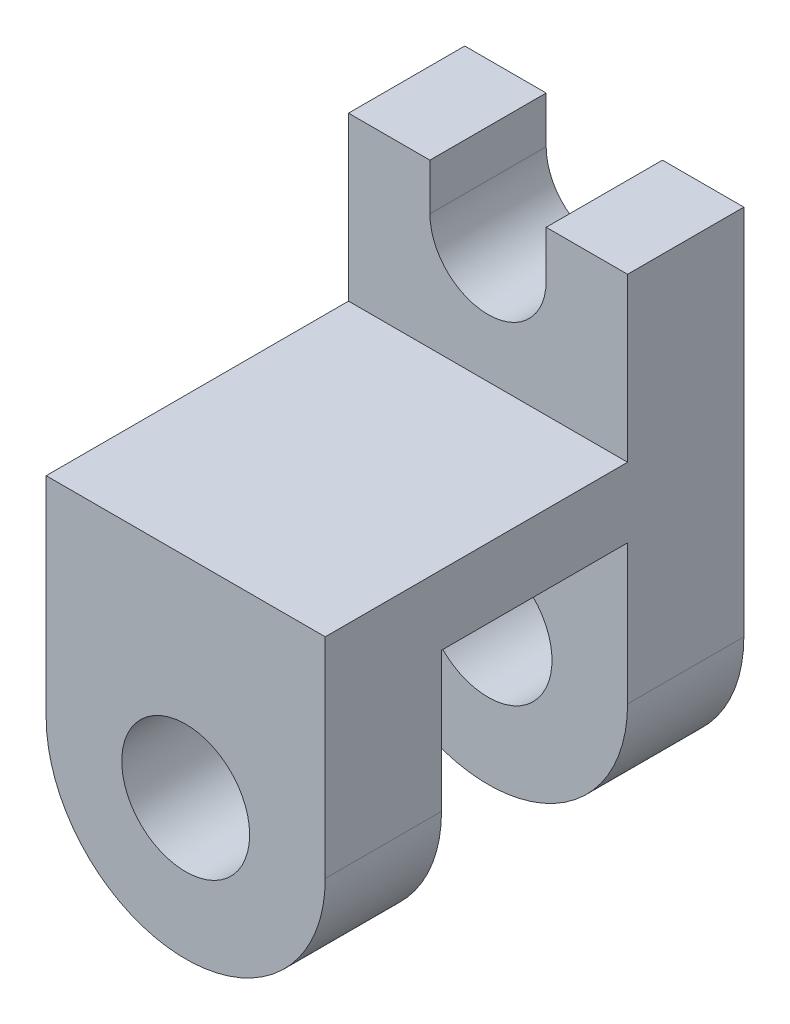
ISO-10303-21;
HEADER;
FILE_DESCRIPTION(('STEP AP214'),'2;1');
FILE_NAME('part.step','',(''),(''),'','','');
FILE_SCHEMA(('AUTOMOTIVE_DESIGN { 1 0 10303 214 1 1 1 1 }'));
ENDSEC;
DATA;
#1=APPLICATION_CONTEXT('core data for automotive mechanical design processes');
#2=APPLICATION_PROTOCOL_DEFINITION('international standard','automotive_design',2000,#1);
#3=PRODUCT_CONTEXT('',#1,'mechanical');
#4=PRODUCT('Part','Part','',(#3));
#5=PRODUCT_RELATED_PRODUCT_CATEGORY('part','',(#4));
#6=PRODUCT_DEFINITION_FORMATION('','',#4);
#7=PRODUCT_DEFINITION_CONTEXT('part definition',#1,'design');
#8=PRODUCT_DEFINITION('design','',#6,#7);
#9=PRODUCT_DEFINITION_SHAPE('','',#8);
#10=(LENGTH_UNIT() NAMED_UNIT(*) SI_UNIT(.MILLI.,.METRE.));
#11=(NAMED_UNIT(*) PLANE_ANGLE_UNIT() SI_UNIT($,.RADIAN.));
#12=(NAMED_UNIT(*) SI_UNIT($,.STERADIAN.) SOLID_ANGLE_UNIT());
#13=UNCERTAINTY_MEASURE_WITH_UNIT(LENGTH_MEASURE(1.E-05),#10,'distance_accuracy_value','');
#14=(GEOMETRIC_REPRESENTATION_CONTEXT(3) GLOBAL_UNCERTAINTY_ASSIGNED_CONTEXT((#13)) GLOBAL_UNIT_ASSIGNED_CONTEXT((#10,
#11,#12)) REPRESENTATION_CONTEXT('',''));
#15=CARTESIAN_POINT('',(0.,0.,0.));
#16=DIRECTION('',(0.,0.,1.));
#17=DIRECTION('',(1.,0.,0.));
#18=AXIS2_PLACEMENT_3D('',#15,#16,#17);
#19=CARTESIAN_POINT('',(-24.,36.,-20.));
#20=DIRECTION('',(0.,1.,0.));
#21=DIRECTION('',(0.,0.,1.));
#22=AXIS2_PLACEMENT_3D('',#19,#20,#21);
#23=PLANE('',#22);
#24=DIRECTION('',(0.,0.,1.));
#25=VECTOR('',#24,1.);
#26=CARTESIAN_POINT('',(24.,36.,-20.));
#27=LINE('',#26,#25);
#28=CARTESIAN_POINT('',(24.,36.,-52.));
#29=VERTEX_POINT('',#28);
#30=CARTESIAN_POINT('',(24.,36.,0.));
#31=VERTEX_POINT('',#30);
#32=EDGE_CURVE('E263',#29,#31,#27,.T.);
#33=ORIENTED_EDGE('',*,*,#32,.F.);
#34=DIRECTION('',(-1.,0.,0.));
#35=VECTOR('',#34,1.);
#36=CARTESIAN_POINT('',(-24.,36.,-52.));
#37=LINE('',#36,#35);
#38=CARTESIAN_POINT('',(-24.,36.,-52.));
#39=VERTEX_POINT('',#38);
#40=EDGE_CURVE('E188',#29,#39,#37,.T.);
#41=ORIENTED_EDGE('',*,*,#40,.T.);
#42=DIRECTION('',(0.,0.,1.));
#43=VECTOR('',#42,1.);
#44=CARTESIAN_POINT('',(-24.,36.,-20.));
#45=LINE('',#44,#43);
#46=CARTESIAN_POINT('',(-24.,36.,0.));
#47=VERTEX_POINT('',#46);
#48=EDGE_CURVE('E53',#39,#47,#45,.T.);
#49=ORIENTED_EDGE('',*,*,#48,.T.);
#50=DIRECTION('',(-1.,0.,0.));
#51=VECTOR('',#50,1.);
#52=CARTESIAN_POINT('',(-24.,36.,0.));
#53=LINE('',#52,#51);
#54=EDGE_CURVE('E260',#31,#47,#53,.T.);
#55=ORIENTED_EDGE('',*,*,#54,.F.);
#56=EDGE_LOOP('',(#33,#41,#49,#55));
#57=FACE_BOUND('',#56,.T.);
#58=ADVANCED_FACE('F44',(#57),#23,.T.);
#59=CARTESIAN_POINT('',(0.,0.,-20.));
#60=DIRECTION('',(0.,0.,1.));
#61=DIRECTION('',(1.,0.,0.));
#62=AXIS2_PLACEMENT_3D('',#59,#60,#61);
#63=CYLINDRICAL_SURFACE('',#62,24.);
#64=CARTESIAN_POINT('',(0.,0.,0.));
#65=DIRECTION('',(0.,0.,1.));
#66=DIRECTION('',(1.,0.,0.));
#67=AXIS2_PLACEMENT_3D('',#64,#65,#66);
#68=CIRCLE('',#67,24.);
#69=CARTESIAN_POINT('',(-24.,0.,0.));
#70=VERTEX_POINT('',#69);
#71=CARTESIAN_POINT('',(24.,0.,0.));
#72=VERTEX_POINT('',#71);
#73=EDGE_CURVE('E243',#70,#72,#68,.T.);
#74=ORIENTED_EDGE('',*,*,#73,.F.);
#75=DIRECTION('',(0.,0.,1.));
#76=VECTOR('',#75,1.);
#77=CARTESIAN_POINT('',(-24.,0.,-20.));
#78=LINE('',#77,#76);
#79=CARTESIAN_POINT('',(-24.,0.,-20.));
#80=VERTEX_POINT('',#79);
#81=EDGE_CURVE('E11',#80,#70,#78,.T.);
#82=ORIENTED_EDGE('',*,*,#81,.F.);
#83=CARTESIAN_POINT('',(0.,0.,-20.));
#84=DIRECTION('',(0.,0.,1.));
#85=DIRECTION('',(1.,0.,0.));
#86=AXIS2_PLACEMENT_3D('',#83,#84,#85);
#87=CIRCLE('',#86,24.);
#88=CARTESIAN_POINT('',(24.,0.,-20.));
#89=VERTEX_POINT('',#88);
#90=EDGE_CURVE('E244',#80,#89,#87,.T.);
#91=ORIENTED_EDGE('',*,*,#90,.T.);
#92=DIRECTION('',(0.,0.,1.));
#93=VECTOR('',#92,1.);
#94=CARTESIAN_POINT('',(24.,0.,-20.));
#95=LINE('',#94,#93);
#96=EDGE_CURVE('E253',#89,#72,#95,.T.);
#97=ORIENTED_EDGE('',*,*,#96,.T.);
#98=EDGE_LOOP('',(#74,#82,#91,#97));
#99=FACE_BOUND('',#98,.T.);
#100=ADVANCED_FACE('F50',(#99),#63,.T.);
#101=CARTESIAN_POINT('',(-24.,0.,-20.));
#102=DIRECTION('',(-1.,0.,0.));
#103=DIRECTION('',(0.,0.,1.));
#104=AXIS2_PLACEMENT_3D('',#101,#102,#103);
#105=PLANE('',#104);
#106=DIRECTION('',(0.,-1.,0.));
#107=VECTOR('',#106,1.);
#108=CARTESIAN_POINT('',(-24.,0.,0.));
#109=LINE('',#108,#107);
#110=EDGE_CURVE('E247',#47,#70,#109,.T.);
#111=ORIENTED_EDGE('',*,*,#110,.F.);
#112=ORIENTED_EDGE('',*,*,#48,.F.);
#113=DIRECTION('',(0.,1.,0.));
#114=VECTOR('',#113,1.);
#115=CARTESIAN_POINT('',(-24.,64.,-52.));
#116=LINE('',#115,#114);
#117=CARTESIAN_POINT('',(-24.,64.,-52.));
#118=VERTEX_POINT('',#117);
#119=EDGE_CURVE('E64',#39,#118,#116,.T.);
#120=ORIENTED_EDGE('',*,*,#119,.T.);
#121=DIRECTION('',(0.,0.,-1.));
#122=VECTOR('',#121,1.);
#123=CARTESIAN_POINT('',(-24.,64.,-52.));
#124=LINE('',#123,#122);
#125=CARTESIAN_POINT('',(-24.,64.,-72.));
#126=VERTEX_POINT('',#125);
#127=EDGE_CURVE('E202',#118,#126,#124,.T.);
#128=ORIENTED_EDGE('',*,*,#127,.T.);
#129=DIRECTION('',(0.,1.,0.));
#130=VECTOR('',#129,1.);
#131=CARTESIAN_POINT('',(-24.,36.,-72.));
#132=LINE('',#131,#130);
#133=CARTESIAN_POINT('',(-24.,0.,-72.));
#134=VERTEX_POINT('',#133);
#135=EDGE_CURVE('E214',#134,#126,#132,.T.);
#136=ORIENTED_EDGE('',*,*,#135,.F.);
#137=DIRECTION('',(0.,0.,1.));
#138=VECTOR('',#137,1.);
#139=CARTESIAN_POINT('',(-24.,0.,-72.));
#140=LINE('',#139,#138);
#141=CARTESIAN_POINT('',(-24.,0.,-52.));
#142=VERTEX_POINT('',#141);
#143=EDGE_CURVE('E230',#134,#142,#140,.T.);
#144=ORIENTED_EDGE('',*,*,#143,.T.);
#145=DIRECTION('',(0.,1.,0.));
#146=VECTOR('',#145,1.);
#147=CARTESIAN_POINT('',(-24.,36.,-52.));
#148=LINE('',#147,#146);
#149=CARTESIAN_POINT('',(-24.,24.,-52.));
#150=VERTEX_POINT('',#149);
#151=EDGE_CURVE('E224',#142,#150,#148,.T.);
#152=ORIENTED_EDGE('',*,*,#151,.T.);
#153=DIRECTION('',(0.,0.,1.));
#154=VECTOR('',#153,1.);
#155=CARTESIAN_POINT('',(-24.,24.,-20.));
#156=LINE('',#155,#154);
#157=CARTESIAN_POINT('',(-24.,24.,-20.));
#158=VERTEX_POINT('',#157);
#159=EDGE_CURVE('E236',#150,#158,#156,.T.);
#160=ORIENTED_EDGE('',*,*,#159,.T.);
#161=DIRECTION('',(0.,-1.,0.));
#162=VECTOR('',#161,1.);
#163=CARTESIAN_POINT('',(-24.,0.,-20.));
#164=LINE('',#163,#162);
#165=EDGE_CURVE('E246',#158,#80,#164,.T.);
#166=ORIENTED_EDGE('',*,*,#165,.T.);
#167=ORIENTED_EDGE('',*,*,#81,.T.);
#168=EDGE_LOOP('',(#111,#112,#120,#128,#136,#144,#152,#160,#166,#167));
#169=FACE_BOUND('',#168,.T.);
#170=ADVANCED_FACE('F276',(#169),#105,.T.);
#171=CARTESIAN_POINT('',(24.,0.,-20.));
#172=DIRECTION('',(1.,0.,0.));
#173=DIRECTION('',(0.,0.,-1.));
#174=AXIS2_PLACEMENT_3D('',#171,#172,#173);
#175=PLANE('',#174);
#176=DIRECTION('',(0.,1.,0.));
#177=VECTOR('',#176,1.);
#178=CARTESIAN_POINT('',(24.,0.,0.));
#179=LINE('',#178,#177);
#180=EDGE_CURVE('E255',#72,#31,#179,.T.);
#181=ORIENTED_EDGE('',*,*,#180,.F.);
#182=ORIENTED_EDGE('',*,*,#96,.F.);
#183=DIRECTION('',(0.,1.,0.));
#184=VECTOR('',#183,1.);
#185=CARTESIAN_POINT('',(24.,0.,-20.));
#186=LINE('',#185,#184);
#187=CARTESIAN_POINT('',(24.,24.,-20.));
#188=VERTEX_POINT('',#187);
#189=EDGE_CURVE('E241',#89,#188,#186,.T.);
#190=ORIENTED_EDGE('',*,*,#189,.T.);
#191=DIRECTION('',(0.,0.,-1.));
#192=VECTOR('',#191,1.);
#193=CARTESIAN_POINT('',(24.,24.,-52.));
#194=LINE('',#193,#192);
#195=CARTESIAN_POINT('',(24.,24.,-52.));
#196=VERTEX_POINT('',#195);
#197=EDGE_CURVE('E68',#188,#196,#194,.T.);
#198=ORIENTED_EDGE('',*,*,#197,.T.);
#199=DIRECTION('',(0.,-1.,0.));
#200=VECTOR('',#199,1.);
#201=CARTESIAN_POINT('',(24.,0.,-52.));
#202=LINE('',#201,#200);
#203=CARTESIAN_POINT('',(24.,0.,-52.));
#204=VERTEX_POINT('',#203);
#205=EDGE_CURVE('E216',#196,#204,#202,.T.);
#206=ORIENTED_EDGE('',*,*,#205,.T.);
#207=DIRECTION('',(0.,0.,1.));
#208=VECTOR('',#207,1.);
#209=CARTESIAN_POINT('',(24.,0.,-72.));
#210=LINE('',#209,#208);
#211=CARTESIAN_POINT('',(24.,0.,-72.));
#212=VERTEX_POINT('',#211);
#213=EDGE_CURVE('E219',#212,#204,#210,.T.);
#214=ORIENTED_EDGE('',*,*,#213,.F.);
#215=DIRECTION('',(0.,-1.,0.));
#216=VECTOR('',#215,1.);
#217=CARTESIAN_POINT('',(24.,0.,-72.));
#218=LINE('',#217,#216);
#219=CARTESIAN_POINT('',(24.,64.,-72.));
#220=VERTEX_POINT('',#219);
#221=EDGE_CURVE('E217',#220,#212,#218,.T.);
#222=ORIENTED_EDGE('',*,*,#221,.F.);
#223=DIRECTION('',(0.,0.,-1.));
#224=VECTOR('',#223,1.);
#225=CARTESIAN_POINT('',(24.,64.,-52.));
#226=LINE('',#225,#224);
#227=CARTESIAN_POINT('',(24.,64.,-52.));
#228=VERTEX_POINT('',#227);
#229=EDGE_CURVE('E208',#228,#220,#226,.T.);
#230=ORIENTED_EDGE('',*,*,#229,.F.);
#231=DIRECTION('',(0.,-1.,0.));
#232=VECTOR('',#231,1.);
#233=CARTESIAN_POINT('',(24.,64.,-52.));
#234=LINE('',#233,#232);
#235=EDGE_CURVE('E181',#228,#29,#234,.T.);
#236=ORIENTED_EDGE('',*,*,#235,.T.);
#237=ORIENTED_EDGE('',*,*,#32,.T.);
#238=EDGE_LOOP('',(#181,#182,#190,#198,#206,#214,#222,#230,#236,#237));
#239=FACE_BOUND('',#238,.T.);
#240=ADVANCED_FACE('F271',(#239),#175,.T.);
#241=CARTESIAN_POINT('',(0.,0.,-20.));
#242=DIRECTION('',(0.,0.,1.));
#243=DIRECTION('',(1.,0.,0.));
#244=AXIS2_PLACEMENT_3D('',#241,#242,#243);
#245=PLANE('',#244);
#246=CARTESIAN_POINT('',(0.,0.,-20.));
#247=DIRECTION('',(0.,0.,1.));
#248=DIRECTION('',(1.,0.,0.));
#249=AXIS2_PLACEMENT_3D('',#246,#247,#248);
#250=CIRCLE('',#249,11.);
#251=CARTESIAN_POINT('',(11.,0.,-20.));
#252=VERTEX_POINT('',#251);
#253=EDGE_CURVE('E176',#252,#252,#250,.T.);
#254=ORIENTED_EDGE('',*,*,#253,.T.);
#255=EDGE_LOOP('',(#254));
#256=FACE_BOUND('',#255,.T.);
#257=ORIENTED_EDGE('',*,*,#165,.F.);
#258=DIRECTION('',(1.,0.,0.));
#259=VECTOR('',#258,1.);
#260=CARTESIAN_POINT('',(24.,24.,-20.));
#261=LINE('',#260,#259);
#262=EDGE_CURVE('E234',#158,#188,#261,.T.);
#263=ORIENTED_EDGE('',*,*,#262,.T.);
#264=ORIENTED_EDGE('',*,*,#189,.F.);
#265=ORIENTED_EDGE('',*,*,#90,.F.);
#266=EDGE_LOOP('',(#257,#263,#264,#265));
#267=FACE_BOUND('',#266,.T.);
#268=ADVANCED_FACE('F284',(#256,#267),#245,.F.);
#269=CARTESIAN_POINT('',(0.,0.,0.));
#270=DIRECTION('',(0.,0.,1.));
#271=DIRECTION('',(1.,0.,0.));
#272=AXIS2_PLACEMENT_3D('',#269,#270,#271);
#273=PLANE('',#272);
#274=CARTESIAN_POINT('',(0.,0.,0.));
#275=DIRECTION('',(0.,0.,1.));
#276=DIRECTION('',(1.,0.,0.));
#277=AXIS2_PLACEMENT_3D('',#274,#275,#276);
#278=CIRCLE('',#277,11.);
#279=CARTESIAN_POINT('',(11.,0.,0.));
#280=VERTEX_POINT('',#279);
#281=EDGE_CURVE('E587',#280,#280,#278,.T.);
#282=ORIENTED_EDGE('',*,*,#281,.F.);
#283=EDGE_LOOP('',(#282));
#284=FACE_BOUND('',#283,.T.);
#285=ORIENTED_EDGE('',*,*,#73,.T.);
#286=ORIENTED_EDGE('',*,*,#180,.T.);
#287=ORIENTED_EDGE('',*,*,#54,.T.);
#288=ORIENTED_EDGE('',*,*,#110,.T.);
#289=EDGE_LOOP('',(#285,#286,#287,#288));
#290=FACE_BOUND('',#289,.T.);
#291=ADVANCED_FACE('F274',(#284,#290),#273,.T.);
#292=CARTESIAN_POINT('',(0.,24.,0.));
#293=DIRECTION('',(0.,-1.,0.));
#294=DIRECTION('',(0.,0.,-1.));
#295=AXIS2_PLACEMENT_3D('',#292,#293,#294);
#296=PLANE('',#295);
#297=ORIENTED_EDGE('',*,*,#262,.F.);
#298=ORIENTED_EDGE('',*,*,#159,.F.);
#299=DIRECTION('',(-1.,0.,0.));
#300=VECTOR('',#299,1.);
#301=CARTESIAN_POINT('',(-24.,24.,-52.));
#302=LINE('',#301,#300);
#303=EDGE_CURVE('E233',#196,#150,#302,.T.);
#304=ORIENTED_EDGE('',*,*,#303,.F.);
#305=ORIENTED_EDGE('',*,*,#197,.F.);
#306=EDGE_LOOP('',(#297,#298,#304,#305));
#307=FACE_BOUND('',#306,.T.);
#308=ADVANCED_FACE('F439',(#307),#296,.T.);
#309=CARTESIAN_POINT('',(0.,0.,-52.));
#310=DIRECTION('',(0.,0.,-1.));
#311=DIRECTION('',(-1.,0.,0.));
#312=AXIS2_PLACEMENT_3D('',#309,#310,#311);
#313=PLANE('',#312);
#314=CARTESIAN_POINT('',(0.,0.,-52.));
#315=DIRECTION('',(0.,0.,-1.));
#316=DIRECTION('',(-1.,0.,0.));
#317=AXIS2_PLACEMENT_3D('',#314,#315,#316);
#318=CIRCLE('',#317,11.);
#319=CARTESIAN_POINT('',(-11.,0.,-52.));
#320=VERTEX_POINT('',#319);
#321=EDGE_CURVE('E588',#320,#320,#318,.T.);
#322=ORIENTED_EDGE('',*,*,#321,.T.);
#323=EDGE_LOOP('',(#322));
#324=FACE_BOUND('',#323,.T.);
#325=ORIENTED_EDGE('',*,*,#205,.F.);
#326=ORIENTED_EDGE('',*,*,#303,.T.);
#327=ORIENTED_EDGE('',*,*,#151,.F.);
#328=CARTESIAN_POINT('',(0.,0.,-52.));
#329=DIRECTION('',(0.,0.,-1.));
#330=DIRECTION('',(-1.,0.,0.));
#331=AXIS2_PLACEMENT_3D('',#328,#329,#330);
#332=CIRCLE('',#331,24.);
#333=EDGE_CURVE('E205',#204,#142,#332,.T.);
#334=ORIENTED_EDGE('',*,*,#333,.F.);
#335=EDGE_LOOP('',(#325,#326,#327,#334));
#336=FACE_BOUND('',#335,.T.);
#337=ADVANCED_FACE('F289',(#324,#336),#313,.F.);
#338=CARTESIAN_POINT('',(0.,0.,-72.));
#339=DIRECTION('',(0.,0.,1.));
#340=DIRECTION('',(1.,0.,0.));
#341=AXIS2_PLACEMENT_3D('',#338,#339,#340);
#342=CYLINDRICAL_SURFACE('',#341,24.);
#343=ORIENTED_EDGE('',*,*,#333,.T.);
#344=ORIENTED_EDGE('',*,*,#143,.F.);
#345=CARTESIAN_POINT('',(0.,0.,-72.));
#346=DIRECTION('',(0.,0.,-1.));
#347=DIRECTION('',(-1.,0.,0.));
#348=AXIS2_PLACEMENT_3D('',#345,#346,#347);
#349=CIRCLE('',#348,24.);
#350=EDGE_CURVE('E215',#212,#134,#349,.T.);
#351=ORIENTED_EDGE('',*,*,#350,.F.);
#352=ORIENTED_EDGE('',*,*,#213,.T.);
#353=EDGE_LOOP('',(#343,#344,#351,#352));
#354=FACE_BOUND('',#353,.T.);
#355=ADVANCED_FACE('F288',(#354),#342,.T.);
#356=CARTESIAN_POINT('',(0.,0.,-72.));
#357=DIRECTION('',(0.,0.,-1.));
#358=DIRECTION('',(-1.,0.,0.));
#359=AXIS2_PLACEMENT_3D('',#356,#357,#358);
#360=PLANE('',#359);
#361=CARTESIAN_POINT('',(0.,0.,-72.));
#362=DIRECTION('',(0.,0.,-1.));
#363=DIRECTION('',(-1.,0.,0.));
#364=AXIS2_PLACEMENT_3D('',#361,#362,#363);
#365=CIRCLE('',#364,11.);
#366=CARTESIAN_POINT('',(-11.,0.,-72.));
#367=VERTEX_POINT('',#366);
#368=EDGE_CURVE('E47',#367,#367,#365,.T.);
#369=ORIENTED_EDGE('',*,*,#368,.F.);
#370=EDGE_LOOP('',(#369));
#371=FACE_BOUND('',#370,.T.);
#372=ORIENTED_EDGE('',*,*,#350,.T.);
#373=ORIENTED_EDGE('',*,*,#135,.T.);
#374=DIRECTION('',(1.,0.,0.));
#375=VECTOR('',#374,1.);
#376=CARTESIAN_POINT('',(-10.,64.,-72.));
#377=LINE('',#376,#375);
#378=CARTESIAN_POINT('',(-10.,64.,-72.));
#379=VERTEX_POINT('',#378);
#380=EDGE_CURVE('E177',#126,#379,#377,.T.);
#381=ORIENTED_EDGE('',*,*,#380,.T.);
#382=DIRECTION('',(0.,-1.,0.));
#383=VECTOR('',#382,1.);
#384=CARTESIAN_POINT('',(-10.,56.,-72.));
#385=LINE('',#384,#383);
#386=CARTESIAN_POINT('',(-10.,56.,-72.));
#387=VERTEX_POINT('',#386);
#388=EDGE_CURVE('E172',#379,#387,#385,.T.);
#389=ORIENTED_EDGE('',*,*,#388,.T.);
#390=CARTESIAN_POINT('',(0.,56.,-72.));
#391=DIRECTION('',(0.,0.,1.));
#392=DIRECTION('',(-1.,0.,0.));
#393=AXIS2_PLACEMENT_3D('',#390,#391,#392);
#394=CIRCLE('',#393,10.);
#395=CARTESIAN_POINT('',(10.,56.,-72.));
#396=VERTEX_POINT('',#395);
#397=EDGE_CURVE('E195',#387,#396,#394,.T.);
#398=ORIENTED_EDGE('',*,*,#397,.T.);
#399=DIRECTION('',(0.,1.,0.));
#400=VECTOR('',#399,1.);
#401=CARTESIAN_POINT('',(10.,56.,-72.));
#402=LINE('',#401,#400);
#403=CARTESIAN_POINT('',(10.,64.,-72.));
#404=VERTEX_POINT('',#403);
#405=EDGE_CURVE('E153',#396,#404,#402,.T.);
#406=ORIENTED_EDGE('',*,*,#405,.T.);
#407=DIRECTION('',(1.,0.,0.));
#408=VECTOR('',#407,1.);
#409=CARTESIAN_POINT('',(10.,64.,-72.));
#410=LINE('',#409,#408);
#411=EDGE_CURVE('E198',#404,#220,#410,.T.);
#412=ORIENTED_EDGE('',*,*,#411,.T.);
#413=ORIENTED_EDGE('',*,*,#221,.T.);
#414=EDGE_LOOP('',(#372,#373,#381,#389,#398,#406,#412,#413));
#415=FACE_BOUND('',#414,.T.);
#416=ADVANCED_FACE('F298',(#371,#415),#360,.T.);
#417=CARTESIAN_POINT('',(0.,56.,-52.));
#418=DIRECTION('',(0.,0.,-1.));
#419=DIRECTION('',(-1.,0.,0.));
#420=AXIS2_PLACEMENT_3D('',#417,#418,#419);
#421=CYLINDRICAL_SURFACE('',#420,10.);
#422=ORIENTED_EDGE('',*,*,#397,.F.);
#423=DIRECTION('',(0.,0.,-1.));
#424=VECTOR('',#423,1.);
#425=CARTESIAN_POINT('',(-10.,56.,-52.));
#426=LINE('',#425,#424);
#427=CARTESIAN_POINT('',(-10.,56.,-52.));
#428=VERTEX_POINT('',#427);
#429=EDGE_CURVE('E174',#428,#387,#426,.T.);
#430=ORIENTED_EDGE('',*,*,#429,.F.);
#431=CARTESIAN_POINT('',(0.,56.,-52.));
#432=DIRECTION('',(0.,0.,1.));
#433=DIRECTION('',(-1.,0.,0.));
#434=AXIS2_PLACEMENT_3D('',#431,#432,#433);
#435=CIRCLE('',#434,10.);
#436=CARTESIAN_POINT('',(10.,56.,-52.));
#437=VERTEX_POINT('',#436);
#438=EDGE_CURVE('E164',#428,#437,#435,.T.);
#439=ORIENTED_EDGE('',*,*,#438,.T.);
#440=DIRECTION('',(0.,0.,-1.));
#441=VECTOR('',#440,1.);
#442=CARTESIAN_POINT('',(10.,56.,-52.));
#443=LINE('',#442,#441);
#444=EDGE_CURVE('E146',#437,#396,#443,.T.);
#445=ORIENTED_EDGE('',*,*,#444,.T.);
#446=EDGE_LOOP('',(#422,#430,#439,#445));
#447=FACE_BOUND('',#446,.T.);
#448=ADVANCED_FACE('F173',(#447),#421,.F.);
#449=CARTESIAN_POINT('',(-10.,56.,-52.));
#450=DIRECTION('',(1.,0.,0.));
#451=DIRECTION('',(0.,0.,-1.));
#452=AXIS2_PLACEMENT_3D('',#449,#450,#451);
#453=PLANE('',#452);
#454=ORIENTED_EDGE('',*,*,#388,.F.);
#455=DIRECTION('',(0.,0.,-1.));
#456=VECTOR('',#455,1.);
#457=CARTESIAN_POINT('',(-10.,64.,-52.));
#458=LINE('',#457,#456);
#459=CARTESIAN_POINT('',(-10.,64.,-52.));
#460=VERTEX_POINT('',#459);
#461=EDGE_CURVE('E201',#460,#379,#458,.T.);
#462=ORIENTED_EDGE('',*,*,#461,.F.);
#463=DIRECTION('',(0.,-1.,0.));
#464=VECTOR('',#463,1.);
#465=CARTESIAN_POINT('',(-10.,56.,-52.));
#466=LINE('',#465,#464);
#467=EDGE_CURVE('E157',#460,#428,#466,.T.);
#468=ORIENTED_EDGE('',*,*,#467,.T.);
#469=ORIENTED_EDGE('',*,*,#429,.T.);
#470=EDGE_LOOP('',(#454,#462,#468,#469));
#471=FACE_BOUND('',#470,.T.);
#472=ADVANCED_FACE('F296',(#471),#453,.T.);
#473=CARTESIAN_POINT('',(-10.,64.,-52.));
#474=DIRECTION('',(0.,1.,0.));
#475=DIRECTION('',(0.,0.,1.));
#476=AXIS2_PLACEMENT_3D('',#473,#474,#475);
#477=PLANE('',#476);
#478=ORIENTED_EDGE('',*,*,#380,.F.);
#479=ORIENTED_EDGE('',*,*,#127,.F.);
#480=DIRECTION('',(1.,0.,0.));
#481=VECTOR('',#480,1.);
#482=CARTESIAN_POINT('',(-10.,64.,-52.));
#483=LINE('',#482,#481);
#484=EDGE_CURVE('E190',#118,#460,#483,.T.);
#485=ORIENTED_EDGE('',*,*,#484,.T.);
#486=ORIENTED_EDGE('',*,*,#461,.T.);
#487=EDGE_LOOP('',(#478,#479,#485,#486));
#488=FACE_BOUND('',#487,.T.);
#489=ADVANCED_FACE('F304',(#488),#477,.T.);
#490=CARTESIAN_POINT('',(10.,64.,-52.));
#491=DIRECTION('',(0.,1.,0.));
#492=DIRECTION('',(0.,0.,1.));
#493=AXIS2_PLACEMENT_3D('',#490,#491,#492);
#494=PLANE('',#493);
#495=ORIENTED_EDGE('',*,*,#411,.F.);
#496=DIRECTION('',(0.,0.,-1.));
#497=VECTOR('',#496,1.);
#498=CARTESIAN_POINT('',(10.,64.,-52.));
#499=LINE('',#498,#497);
#500=CARTESIAN_POINT('',(10.,64.,-52.));
#501=VERTEX_POINT('',#500);
#502=EDGE_CURVE('E158',#501,#404,#499,.T.);
#503=ORIENTED_EDGE('',*,*,#502,.F.);
#504=DIRECTION('',(1.,0.,0.));
#505=VECTOR('',#504,1.);
#506=CARTESIAN_POINT('',(10.,64.,-52.));
#507=LINE('',#506,#505);
#508=EDGE_CURVE('E166',#501,#228,#507,.T.);
#509=ORIENTED_EDGE('',*,*,#508,.T.);
#510=ORIENTED_EDGE('',*,*,#229,.T.);
#511=EDGE_LOOP('',(#495,#503,#509,#510));
#512=FACE_BOUND('',#511,.T.);
#513=ADVANCED_FACE('F293',(#512),#494,.T.);
#514=CARTESIAN_POINT('',(10.,56.,-52.));
#515=DIRECTION('',(-1.,0.,0.));
#516=DIRECTION('',(0.,0.,1.));
#517=AXIS2_PLACEMENT_3D('',#514,#515,#516);
#518=PLANE('',#517);
#519=ORIENTED_EDGE('',*,*,#405,.F.);
#520=ORIENTED_EDGE('',*,*,#444,.F.);
#521=DIRECTION('',(0.,1.,0.));
#522=VECTOR('',#521,1.);
#523=CARTESIAN_POINT('',(10.,56.,-52.));
#524=LINE('',#523,#522);
#525=EDGE_CURVE('E151',#437,#501,#524,.T.);
#526=ORIENTED_EDGE('',*,*,#525,.T.);
#527=ORIENTED_EDGE('',*,*,#502,.T.);
#528=EDGE_LOOP('',(#519,#520,#526,#527));
#529=FACE_BOUND('',#528,.T.);
#530=ADVANCED_FACE('F147',(#529),#518,.T.);
#531=CARTESIAN_POINT('',(0.,56.,-52.));
#532=DIRECTION('',(0.,0.,-1.));
#533=DIRECTION('',(-1.,0.,0.));
#534=AXIS2_PLACEMENT_3D('',#531,#532,#533);
#535=PLANE('',#534);
#536=ORIENTED_EDGE('',*,*,#438,.F.);
#537=ORIENTED_EDGE('',*,*,#467,.F.);
#538=ORIENTED_EDGE('',*,*,#484,.F.);
#539=ORIENTED_EDGE('',*,*,#119,.F.);
#540=ORIENTED_EDGE('',*,*,#40,.F.);
#541=ORIENTED_EDGE('',*,*,#235,.F.);
#542=ORIENTED_EDGE('',*,*,#508,.F.);
#543=ORIENTED_EDGE('',*,*,#525,.F.);
#544=EDGE_LOOP('',(#536,#537,#538,#539,#540,#541,#542,#543));
#545=FACE_BOUND('',#544,.T.);
#546=ADVANCED_FACE('F162',(#545),#535,.F.);
#547=CARTESIAN_POINT('',(0.,0.,-99.));
#548=DIRECTION('',(0.,0.,1.));
#549=DIRECTION('',(1.,0.,0.));
#550=AXIS2_PLACEMENT_3D('',#547,#548,#549);
#551=CYLINDRICAL_SURFACE('',#550,11.);
#552=ORIENTED_EDGE('',*,*,#368,.T.);
#553=EDGE_LOOP('',(#552));
#554=FACE_BOUND('',#553,.T.);
#555=ORIENTED_EDGE('',*,*,#321,.F.);
#556=EDGE_LOOP('',(#555));
#557=FACE_BOUND('',#556,.T.);
#558=ADVANCED_FACE('F384',(#554,#557),#551,.F.);
#559=ORIENTED_EDGE('',*,*,#281,.T.);
#560=EDGE_LOOP('',(#559));
#561=FACE_BOUND('',#560,.T.);
#562=ORIENTED_EDGE('',*,*,#253,.F.);
#563=EDGE_LOOP('',(#562));
#564=FACE_BOUND('',#563,.T.);
#565=ADVANCED_FACE('F411',(#561,#564),#551,.F.);
#566=CLOSED_SHELL('',(#58,#100,#170,#240,#268,#291,#308,#337,#355,#416,#448,#472,#489,#513,#530,
#546,#558,#565));
#567=MANIFOLD_SOLID_BREP('B2',#566);
#568=ADVANCED_BREP_SHAPE_REPRESENTATION('',(#18,#567),#14);
#569=SHAPE_DEFINITION_REPRESENTATION(#9,#568);
ENDSEC;
END-ISO-10303-21;
